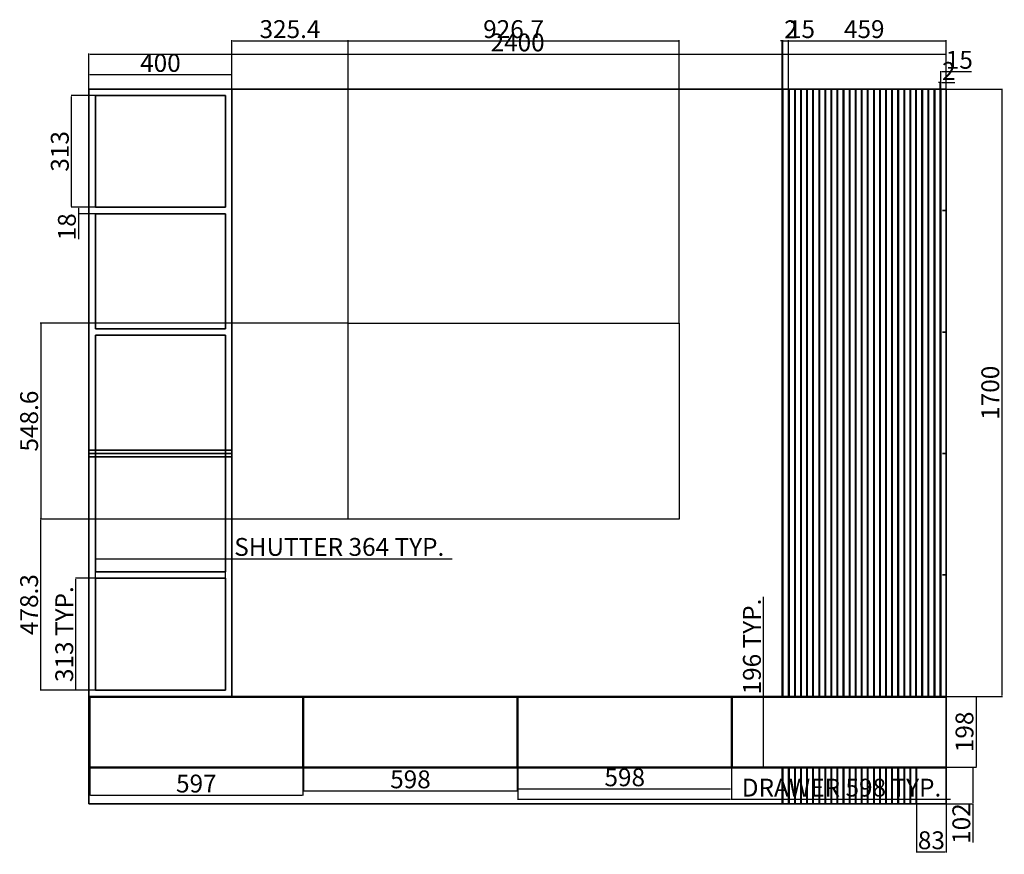
# Model space of a CAD drawing. Units: millimetres. Extents: x 805 to 3562, y 495 to 2830.
import ezdxf

# ---------------------------------------------------------------- set-up
doc = ezdxf.new("R2010")
doc.units = ezdxf.units.MM
for name, color, linetype, lineweight in [('A-ANNO-DIMS', 2, 'Continuous', 18), ('A-EQPM', 8, 'Continuous', 25), ('A-FURN', 7, 'Continuous', 35), ('A-FURN-PATT', 8, 'Continuous', 13)]:
    doc.layers.add(name, color=color, linetype=linetype, lineweight=lineweight)
doc.styles.get("Standard").update_dxf_attribs({"font": 'arial.ttf'})
doc.dimstyles.new('ISO-25', dxfattribs={"dimtxt": 50, "dimasz": 2.5, "dimexe": 1.25, "dimexo": 0.625, "dimtad": 1, "dimtxsty": 'Standard', "dimcen": 2.5, "dimadec": 0, "dimazin": 0, "dimtfac": 1, "dimtmove": 0, "dimatfit": 3, "dimfxl": 1, "dimarcsym": 0})

# ---------------------------------------------------------------- blocks, each defined once
blk = doc.blocks.new('*D1')
at = {"layer": 'A-ANNO-DIMS', "color": 0, "lineweight": -2, "transparency": 16777216}
for p, q in [((999, 2637.1), (999, 2735.5)), ((1001.5, 2734.2), (3396.5, 2734.2)), ((3399, 2637.1), (3399, 2735.5))]:
    blk.add_line(p, q, dxfattribs=at)
at = {"layer": 'A-ANNO-DIMS', "color": 0, "transparency": 16777216}
for points in [[(1001.5, 2734.6), (1001.5, 2733.8), (999, 2734.2)], [(3396.5, 2734.6), (3396.5, 2733.8), (3399, 2734.2)]]:
    blk.add_solid(points, dxfattribs=at)
at = {"layer": 'Defpoints', "color": 0, "transparency": 16777216}
for p in [(3399, 2734.2), (999, 2636.4), (3399, 2636.4)]:
    blk.add_point(p, dxfattribs=at)
at = {"layer": 'A-ANNO-DIMS', "color": 0, "transparency": 16777216, "insert": (2199, 2760.4), "char_height": 50, "attachment_point": 5}
blk.add_mtext('2400', dxfattribs=at)
blk = doc.blocks.new('*D2')
at = {"layer": 'A-ANNO-DIMS', "color": 0, "lineweight": -2, "transparency": 16777216}
for p, q in [((3384, 2637.1), (3384, 2686.8)), ((3386.5, 2685.6), (3396.5, 2685.6)), ((3399, 2637.1), (3399, 2686.8)), ((3399, 2685.6), (3470, 2685.6))]:
    blk.add_line(p, q, dxfattribs=at)
at = {"layer": 'A-ANNO-DIMS', "color": 0, "transparency": 16777216}
for points in [[(3386.5, 2686), (3386.5, 2685.1), (3384, 2685.6)], [(3396.5, 2686), (3396.5, 2685.1), (3399, 2685.6)]]:
    blk.add_solid(points, dxfattribs=at)
at = {"layer": 'Defpoints', "color": 0, "transparency": 16777216}
for p in [(3399, 2685.6), (3384, 2636.4), (3399, 2636.4)]:
    blk.add_point(p, dxfattribs=at)
at = {"layer": 'A-ANNO-DIMS', "color": 0, "transparency": 16777216, "insert": (3435.7, 2711.7), "char_height": 50, "attachment_point": 5}
blk.add_mtext('15', dxfattribs=at)
blk = doc.blocks.new('*D3')
at = {"layer": 'A-ANNO-DIMS', "color": 0, "lineweight": -2, "transparency": 16777216}
for p, q in [((3379.5, 2654.8), (3377, 2654.8)), ((3382, 2637.1), (3382, 2656.1)), ((3382, 2654.8), (3384, 2654.8)), ((3384, 2637.1), (3384, 2656.1)), ((3386.5, 2654.8), (3423.3, 2654.8))]:
    blk.add_line(p, q, dxfattribs=at)
at = {"layer": 'A-ANNO-DIMS', "color": 0, "transparency": 16777216}
for points in [[(3379.5, 2655.2), (3379.5, 2654.4), (3382, 2654.8)], [(3386.5, 2655.2), (3386.5, 2654.4), (3384, 2654.8)]]:
    blk.add_solid(points, dxfattribs=at)
at = {"layer": 'Defpoints', "color": 0, "transparency": 16777216}
for p in [(3384, 2654.8), (3382, 2636.4), (3384, 2636.4)]:
    blk.add_point(p, dxfattribs=at)
at = {"layer": 'A-ANNO-DIMS', "color": 0, "transparency": 16777216, "insert": (3406.2, 2680.5), "char_height": 50, "attachment_point": 5}
blk.add_mtext('2', dxfattribs=at)
blk = doc.blocks.new('*D4')
at = {"layer": 'A-ANNO-DIMS', "color": 0, "lineweight": -2, "transparency": 16777216}
for p, q in [((3399.6, 2636.4), (3556.2, 2636.4)), ((3555, 2633.9), (3555, 938.9)), ((3399.6, 936.4), (3556.2, 936.4))]:
    blk.add_line(p, q, dxfattribs=at)
at = {"layer": 'A-ANNO-DIMS', "color": 0, "transparency": 16777216}
for points in [[(3554.6, 2633.9), (3555.4, 2633.9), (3555, 2636.4)], [(3554.6, 938.9), (3555.4, 938.9), (3555, 936.4)]]:
    blk.add_solid(points, dxfattribs=at)
at = {"layer": 'Defpoints', "color": 0, "transparency": 16777216}
for p in [(3399, 2636.4), (3399, 936.4), (3555, 936.4)]:
    blk.add_point(p, dxfattribs=at)
at = {"layer": 'A-ANNO-DIMS', "color": 0, "transparency": 16777216, "insert": (3528.8, 1786.4), "char_height": 50, "attachment_point": 5, "rotation": 90}
blk.add_mtext('1700', dxfattribs=at)
blk = doc.blocks.new('*D5')
at = {"layer": 'A-ANNO-DIMS', "color": 0, "lineweight": -2, "transparency": 16777216}
for p, q in [((3399.6, 936.4), (3484, 936.4)), ((3482.7, 933.9), (3482.7, 740.9)), ((3399.6, 738.4), (3484, 738.4))]:
    blk.add_line(p, q, dxfattribs=at)
at = {"layer": 'A-ANNO-DIMS', "color": 0, "transparency": 16777216}
for points in [[(3482.3, 933.9), (3483.2, 933.9), (3482.7, 936.4)], [(3482.3, 740.9), (3483.2, 740.9), (3482.7, 738.4)]]:
    blk.add_solid(points, dxfattribs=at)
at = {"layer": 'Defpoints', "color": 0, "transparency": 16777216}
for p in [(3399, 936.4), (3399, 738.4), (3482.7, 738.4)]:
    blk.add_point(p, dxfattribs=at)
at = {"layer": 'A-ANNO-DIMS', "color": 0, "transparency": 16777216, "insert": (3456.6, 837.4), "char_height": 50, "attachment_point": 5, "rotation": 90}
blk.add_mtext('198', dxfattribs=at)
blk = doc.blocks.new('*D6')
at = {"layer": 'A-ANNO-DIMS', "color": 0, "lineweight": -2, "transparency": 16777216}
for p, q in [((3399.6, 738.4), (3475.2, 738.4)), ((3473.9, 735.9), (3473.9, 638.9)), ((3399.6, 636.4), (3475.2, 636.4)), ((3473.9, 636.4), (3473.9, 527.4))]:
    blk.add_line(p, q, dxfattribs=at)
at = {"layer": 'A-ANNO-DIMS', "color": 0, "transparency": 16777216}
for points in [[(3473.5, 735.9), (3474.3, 735.9), (3473.9, 738.4)], [(3473.5, 638.9), (3474.3, 638.9), (3473.9, 636.4)]]:
    blk.add_solid(points, dxfattribs=at)
at = {"layer": 'Defpoints', "color": 0, "transparency": 16777216}
for p in [(3399, 738.4), (3399, 636.4), (3473.9, 636.4)]:
    blk.add_point(p, dxfattribs=at)
at = {"layer": 'A-ANNO-DIMS', "color": 0, "transparency": 16777216, "insert": (3447.8, 580.7), "char_height": 50, "attachment_point": 5, "rotation": 90}
blk.add_mtext('102', dxfattribs=at)
blk = doc.blocks.new('*D7')
at = {"layer": 'A-ANNO-DIMS', "color": 0, "lineweight": -2, "transparency": 16777216}
for p, q in [((999, 2637.1), (999, 2678.1)), ((1001.5, 2676.9), (1396.5, 2676.9)), ((1399, 2637.1), (1399, 2678.1))]:
    blk.add_line(p, q, dxfattribs=at)
at = {"layer": 'A-ANNO-DIMS', "color": 0, "transparency": 16777216}
for points in [[(1001.5, 2677.3), (1001.5, 2676.5), (999, 2676.9)], [(1396.5, 2677.3), (1396.5, 2676.5), (1399, 2676.9)]]:
    blk.add_solid(points, dxfattribs=at)
at = {"layer": 'Defpoints', "color": 0, "transparency": 16777216}
for p in [(1399, 2676.9), (999, 2636.4), (1399, 2636.4)]:
    blk.add_point(p, dxfattribs=at)
at = {"layer": 'A-ANNO-DIMS', "color": 0, "transparency": 16777216, "insert": (1199, 2703), "char_height": 50, "attachment_point": 5}
blk.add_mtext('400', dxfattribs=at)
blk = doc.blocks.new('*D8')
at = {"layer": 'A-ANNO-DIMS', "color": 0, "lineweight": -2, "transparency": 16777216}
for p, q in [((1016.3, 2618.4), (948.7, 2618.4)), ((949.9, 2307.9), (949.9, 2615.9)), ((1016.3, 2305.4), (948.7, 2305.4))]:
    blk.add_line(p, q, dxfattribs=at)
at = {"layer": 'A-ANNO-DIMS', "color": 0, "transparency": 16777216}
for points in [[(949.5, 2615.9), (950.3, 2615.9), (949.9, 2618.4)], [(949.5, 2307.9), (950.3, 2307.9), (949.9, 2305.4)]]:
    blk.add_solid(points, dxfattribs=at)
at = {"layer": 'Defpoints', "color": 0, "transparency": 16777216}
for p in [(949.9, 2618.4), (1017, 2618.4), (1017, 2305.4)]:
    blk.add_point(p, dxfattribs=at)
at = {"layer": 'A-ANNO-DIMS', "color": 0, "transparency": 16777216, "insert": (923.8, 2461.9), "char_height": 50, "attachment_point": 5, "rotation": 90}
blk.add_mtext('313', dxfattribs=at)
blk = doc.blocks.new('*D9')
at = {"layer": 'A-ANNO-DIMS', "color": 0, "lineweight": -2, "transparency": 16777216}
for p, q in [((1001, 737.8), (1001, 658.9)), ((1598, 737.8), (1598, 658.9)), ((1003.5, 660.1), (1595.5, 660.1))]:
    blk.add_line(p, q, dxfattribs=at)
at = {"layer": 'A-ANNO-DIMS', "color": 0, "transparency": 16777216}
for points in [[(1003.5, 660.6), (1003.5, 659.7), (1001, 660.1)], [(1595.5, 660.6), (1595.5, 659.7), (1598, 660.1)]]:
    blk.add_solid(points, dxfattribs=at)
at = {"layer": 'Defpoints', "color": 0, "transparency": 16777216}
for p in [(1001, 738.4), (1598, 738.4), (1598, 660.1)]:
    blk.add_point(p, dxfattribs=at)
at = {"layer": 'A-ANNO-DIMS', "color": 0, "transparency": 16777216, "insert": (1299.5, 686.3), "char_height": 50, "attachment_point": 5}
blk.add_mtext('597', dxfattribs=at)
blk = doc.blocks.new('*D10')
at = {"layer": 'A-ANNO-DIMS', "color": 0, "lineweight": -2, "transparency": 16777216}
for p, q in [((1600, 737.8), (1600, 670.7)), ((2198, 737.8), (2198, 670.7)), ((1602.5, 672), (2195.5, 672))]:
    blk.add_line(p, q, dxfattribs=at)
at = {"layer": 'A-ANNO-DIMS', "color": 0, "transparency": 16777216}
for points in [[(1602.5, 672.4), (1602.5, 671.6), (1600, 672)], [(2195.5, 672.4), (2195.5, 671.6), (2198, 672)]]:
    blk.add_solid(points, dxfattribs=at)
at = {"layer": 'Defpoints', "color": 0, "transparency": 16777216}
for p in [(1600, 738.4), (2198, 738.4), (2198, 672)]:
    blk.add_point(p, dxfattribs=at)
at = {"layer": 'A-ANNO-DIMS', "color": 0, "transparency": 16777216, "insert": (1899, 698.1), "char_height": 50, "attachment_point": 5}
blk.add_mtext('598', dxfattribs=at)
blk = doc.blocks.new('*D11')
at = {"layer": 'A-ANNO-DIMS', "color": 0, "lineweight": -2, "transparency": 16777216}
for p, q in [((2200, 737.8), (2200, 676.4)), ((2798, 737.8), (2798, 676.4)), ((2202.5, 677.6), (2795.5, 677.6))]:
    blk.add_line(p, q, dxfattribs=at)
at = {"layer": 'A-ANNO-DIMS', "color": 0, "transparency": 16777216}
for points in [[(2202.5, 678), (2202.5, 677.2), (2200, 677.6)], [(2795.5, 678), (2795.5, 677.2), (2798, 677.6)]]:
    blk.add_solid(points, dxfattribs=at)
at = {"layer": 'Defpoints', "color": 0, "transparency": 16777216}
for p in [(2200, 738.4), (2798, 738.4), (2798, 677.6)]:
    blk.add_point(p, dxfattribs=at)
at = {"layer": 'A-ANNO-DIMS', "color": 0, "transparency": 16777216, "insert": (2499, 703.8), "char_height": 50, "attachment_point": 5}
blk.add_mtext('598', dxfattribs=at)
blk = doc.blocks.new('*D12')
at = {"layer": 'A-ANNO-DIMS', "color": 0, "lineweight": -2, "transparency": 16777216}
for p, q in [((1016.3, 2305.4), (968.5, 2305.4)), ((969.8, 2302.9), (969.8, 2289.9)), ((1016.3, 2287.4), (968.5, 2287.4)), ((969.8, 2287.4), (969.8, 2216.7))]:
    blk.add_line(p, q, dxfattribs=at)
at = {"layer": 'A-ANNO-DIMS', "color": 0, "transparency": 16777216}
for points in [[(969.3, 2302.9), (970.2, 2302.9), (969.8, 2305.4)], [(969.3, 2289.9), (970.2, 2289.9), (969.8, 2287.4)]]:
    blk.add_solid(points, dxfattribs=at)
at = {"layer": 'Defpoints', "color": 0, "transparency": 16777216}
for p in [(1017, 2305.4), (969.8, 2287.4), (1017, 2287.4)]:
    blk.add_point(p, dxfattribs=at)
at = {"layer": 'A-ANNO-DIMS', "color": 0, "transparency": 16777216, "insert": (943.6, 2250.8), "char_height": 50, "attachment_point": 5, "rotation": 90}
blk.add_mtext('18', dxfattribs=at)
blk = doc.blocks.new('SHUTTER-364x313')
for p, q in [((0, 313), (0, 0)), ((0, 313), (364, 313)), ((364, 313), (364, 0)), ((364, 0), (0, 0))]:
    blk.add_line(p, q)
blk = doc.blocks.new('DRAWER-600')
for p, q in [((0, 196), (0, 0)), ((0, 196), (598, 196)), ((598, 196), (598, 0)), ((0, 0), (598, 0))]:
    blk.add_line(p, q)
blk = doc.blocks.new('*D15')
at = {"layer": 'A-ANNO-DIMS', "color": 0, "lineweight": -2, "transparency": 16777216}
for p, q in [((1017, 1268.1), (1017, 1323.3)), ((1381, 1268.1), (1381, 1323.3)), ((1019.5, 1322), (1378.5, 1322)), ((1381, 1322), (2016, 1322))]:
    blk.add_line(p, q, dxfattribs=at)
at = {"layer": 'A-ANNO-DIMS', "color": 0, "transparency": 16777216}
for points in [[(1019.5, 1322.4), (1019.5, 1321.6), (1017, 1322)], [(1378.5, 1322.4), (1378.5, 1321.6), (1381, 1322)]]:
    blk.add_solid(points, dxfattribs=at)
at = {"layer": 'Defpoints', "color": 0, "transparency": 16777216}
for p in [(1381, 1322), (1017, 1267.4), (1381, 1267.4)]:
    blk.add_point(p, dxfattribs=at)
at = {"layer": 'A-ANNO-DIMS', "color": 0, "transparency": 16777216, "insert": (1699.7, 1348.5), "char_height": 50, "attachment_point": 5}
blk.add_mtext('SHUTTER 364 TYP.', dxfattribs=at)
blk = doc.blocks.new('*D16')
at = {"layer": 'A-ANNO-DIMS', "color": 0, "lineweight": -2, "transparency": 16777216}
for p, q in [((1016.3, 1267.4), (961.1, 1267.4)), ((962.4, 956.9), (962.4, 1264.9)), ((1016.3, 954.4), (961.1, 954.4))]:
    blk.add_line(p, q, dxfattribs=at)
at = {"layer": 'A-ANNO-DIMS', "color": 0, "transparency": 16777216}
for points in [[(961.9, 1264.9), (962.8, 1264.9), (962.4, 1267.4)], [(961.9, 956.9), (962.8, 956.9), (962.4, 954.4)]]:
    blk.add_solid(points, dxfattribs=at)
at = {"layer": 'Defpoints', "color": 0, "transparency": 16777216}
for p in [(962.4, 1267.4), (1017, 1267.4), (1017, 954.4)]:
    blk.add_point(p, dxfattribs=at)
at = {"layer": 'A-ANNO-DIMS', "color": 0, "transparency": 16777216, "insert": (936.2, 1110.9), "char_height": 50, "attachment_point": 5, "rotation": 90}
blk.add_mtext('313 TYP.', dxfattribs=at)
blk = doc.blocks.new('*D17')
at = {"layer": 'A-ANNO-DIMS', "color": 0, "lineweight": -2, "transparency": 16777216}
for p, q in [((2200, 737.8), (2200, 647.5)), ((2798, 737.8), (2798, 647.5)), ((2202.5, 648.7), (2795.5, 648.7)), ((2798, 648.7), (3411.3, 648.7))]:
    blk.add_line(p, q, dxfattribs=at)
at = {"layer": 'A-ANNO-DIMS', "color": 0, "transparency": 16777216}
for points in [[(2202.5, 649.1), (2202.5, 648.3), (2200, 648.7)], [(2795.5, 649.1), (2795.5, 648.3), (2798, 648.7)]]:
    blk.add_solid(points, dxfattribs=at)
at = {"layer": 'Defpoints', "color": 0, "transparency": 16777216}
for p in [(2200, 738.4), (2798, 738.4), (2798, 648.7)]:
    blk.add_point(p, dxfattribs=at)
at = {"layer": 'A-ANNO-DIMS', "color": 0, "transparency": 16777216, "insert": (3105.9, 674.9), "char_height": 50, "attachment_point": 5}
blk.add_mtext('DRAWER 598 TYP.', dxfattribs=at)
blk = doc.blocks.new('*D18')
at = {"layer": 'A-ANNO-DIMS', "color": 0, "lineweight": -2, "transparency": 16777216}
for p, q in [((2887.7, 934.4), (2887.7, 1215.7)), ((2798.6, 934.4), (2888.9, 934.4)), ((2887.7, 740.9), (2887.7, 931.9)), ((2798.6, 738.4), (2888.9, 738.4))]:
    blk.add_line(p, q, dxfattribs=at)
at = {"layer": 'A-ANNO-DIMS', "color": 0, "transparency": 16777216}
for points in [[(2887.2, 931.9), (2888.1, 931.9), (2887.7, 934.4)], [(2887.2, 740.9), (2888.1, 740.9), (2887.7, 738.4)]]:
    blk.add_solid(points, dxfattribs=at)
at = {"layer": 'Defpoints', "color": 0, "transparency": 16777216}
for p in [(2798, 934.4), (2887.7, 934.4), (2798, 738.4)]:
    blk.add_point(p, dxfattribs=at)
at = {"layer": 'A-ANNO-DIMS', "color": 0, "transparency": 16777216, "insert": (2861.5, 1076.3), "char_height": 50, "attachment_point": 5, "rotation": 90}
blk.add_mtext('196 TYP.', dxfattribs=at)
blk = doc.blocks.new('*D19')
at = {"layer": 'A-ANNO-DIMS', "color": 0, "lineweight": -2, "transparency": 16777216}
for p, q in [((1724.4, 1982), (1724.4, 2772.7)), ((1726.9, 2771.4), (2648.6, 2771.4)), ((2651.1, 1982), (2651.1, 2772.7))]:
    blk.add_line(p, q, dxfattribs=at)
at = {"layer": 'A-ANNO-DIMS', "color": 0, "transparency": 16777216}
for points in [[(1726.9, 2771.8), (1726.9, 2771), (1724.4, 2771.4)], [(2648.6, 2771.8), (2648.6, 2771), (2651.1, 2771.4)]]:
    blk.add_solid(points, dxfattribs=at)
at = {"layer": 'Defpoints', "color": 0, "transparency": 16777216}
for p in [(2651.1, 2771.4), (1724.4, 1981.4), (2651.1, 1981.4)]:
    blk.add_point(p, dxfattribs=at)
at = {"layer": 'A-ANNO-DIMS', "color": 0, "transparency": 16777216, "insert": (2187.8, 2797.6), "char_height": 50, "attachment_point": 5}
blk.add_mtext('926.7', dxfattribs=at)
blk = doc.blocks.new('*D20')
at = {"layer": 'A-ANNO-DIMS', "color": 0, "lineweight": -2, "transparency": 16777216}
for p, q in [((1723.8, 1981.4), (862.7, 1981.4)), ((864, 1978.9), (864, 1435.2)), ((1723.8, 1432.7), (862.7, 1432.7))]:
    blk.add_line(p, q, dxfattribs=at)
at = {"layer": 'A-ANNO-DIMS', "color": 0, "transparency": 16777216}
for points in [[(863.5, 1978.9), (864.4, 1978.9), (864, 1981.4)], [(863.5, 1435.2), (864.4, 1435.2), (864, 1432.7)]]:
    blk.add_solid(points, dxfattribs=at)
at = {"layer": 'Defpoints', "color": 0, "transparency": 16777216}
for p in [(1724.4, 1981.4), (864, 1432.7), (1724.4, 1432.7)]:
    blk.add_point(p, dxfattribs=at)
at = {"layer": 'A-ANNO-DIMS', "color": 0, "transparency": 16777216, "insert": (837.8, 1707.1), "char_height": 50, "attachment_point": 5, "rotation": 90}
blk.add_mtext('548.6', dxfattribs=at)
blk = doc.blocks.new('*D21')
at = {"layer": 'A-ANNO-DIMS', "color": 0, "lineweight": -2, "transparency": 16777216}
for p, q in [((1399, 2637.1), (1399, 2772.7)), ((1401.5, 2771.4), (1721.9, 2771.4)), ((1724.4, 1982), (1724.4, 2772.7))]:
    blk.add_line(p, q, dxfattribs=at)
at = {"layer": 'A-ANNO-DIMS', "color": 0, "transparency": 16777216}
for points in [[(1401.5, 2771.8), (1401.5, 2771), (1399, 2771.4)], [(1721.9, 2771.8), (1721.9, 2771), (1724.4, 2771.4)]]:
    blk.add_solid(points, dxfattribs=at)
at = {"layer": 'Defpoints', "color": 0, "transparency": 16777216}
for p in [(1724.4, 2771.4), (1399, 2636.4), (1724.4, 1981.4)]:
    blk.add_point(p, dxfattribs=at)
at = {"layer": 'A-ANNO-DIMS', "color": 0, "transparency": 16777216, "insert": (1561.7, 2797.6), "char_height": 50, "attachment_point": 5}
blk.add_mtext('325.4', dxfattribs=at)
blk = doc.blocks.new('*D22')
at = {"layer": 'A-ANNO-DIMS', "color": 0, "lineweight": -2, "transparency": 16777216}
for p, q in [((1723.8, 1432.7), (862.7, 1432.7)), ((864, 956.9), (864, 1430.2)), ((1380.3, 954.4), (862.7, 954.4))]:
    blk.add_line(p, q, dxfattribs=at)
at = {"layer": 'A-ANNO-DIMS', "color": 0, "transparency": 16777216}
for points in [[(863.5, 1430.2), (864.4, 1430.2), (864, 1432.7)], [(863.5, 956.9), (864.4, 956.9), (864, 954.4)]]:
    blk.add_solid(points, dxfattribs=at)
at = {"layer": 'Defpoints', "color": 0, "transparency": 16777216}
for p in [(864, 1432.7), (1724.4, 1432.7), (1381, 954.4)]:
    blk.add_point(p, dxfattribs=at)
at = {"layer": 'A-ANNO-DIMS', "color": 0, "transparency": 16777216, "insert": (837.8, 1193.6), "char_height": 50, "attachment_point": 5, "rotation": 90}
blk.add_mtext('478.3', dxfattribs=at)
blk = doc.blocks.new('*D23')
at = {"layer": 'A-ANNO-DIMS', "color": 0, "lineweight": -2, "transparency": 16777216}
for p, q in [((2940, 937.1), (2940, 2772.7)), ((2942.5, 2771.4), (3396.5, 2771.4)), ((3399, 937.1), (3399, 2772.7))]:
    blk.add_line(p, q, dxfattribs=at)
at = {"layer": 'A-ANNO-DIMS', "color": 0, "transparency": 16777216}
for points in [[(2942.5, 2771.8), (2942.5, 2771), (2940, 2771.4)], [(3396.5, 2771.8), (3396.5, 2771), (3399, 2771.4)]]:
    blk.add_solid(points, dxfattribs=at)
at = {"layer": 'Defpoints', "color": 0, "transparency": 16777216}
for p in [(3399, 2771.4), (2940, 936.4), (3399, 936.4)]:
    blk.add_point(p, dxfattribs=at)
at = {"layer": 'A-ANNO-DIMS', "color": 0, "transparency": 16777216, "insert": (3169.5, 2797.6), "char_height": 50, "attachment_point": 5}
blk.add_mtext('459', dxfattribs=at)
blk = doc.blocks.new('*D24')
at = {"layer": 'A-ANNO-DIMS', "color": 0, "lineweight": -2, "transparency": 16777216}
for p, q in [((2937.5, 2771.4), (2935, 2771.4)), ((2940, 2637.1), (2940, 2772.7)), ((2940, 2771.4), (2942, 2771.4)), ((2942, 2637.1), (2942, 2772.7)), ((2944.5, 2771.4), (2981.3, 2771.4))]:
    blk.add_line(p, q, dxfattribs=at)
at = {"layer": 'A-ANNO-DIMS', "color": 0, "transparency": 16777216}
for points in [[(2937.5, 2771.8), (2937.5, 2771), (2940, 2771.4)], [(2944.5, 2771.8), (2944.5, 2771), (2942, 2771.4)]]:
    blk.add_solid(points, dxfattribs=at)
at = {"layer": 'Defpoints', "color": 0, "transparency": 16777216}
for p in [(2942, 2771.4), (2940, 2636.4), (2942, 2636.4)]:
    blk.add_point(p, dxfattribs=at)
at = {"layer": 'A-ANNO-DIMS', "color": 0, "transparency": 16777216, "insert": (2964.2, 2797.2), "char_height": 50, "attachment_point": 5}
blk.add_mtext('2', dxfattribs=at)
blk = doc.blocks.new('*D25')
at = {"layer": 'A-ANNO-DIMS', "color": 0, "lineweight": -2, "transparency": 16777216}
for p, q in [((2942, 2637.1), (2942, 2772.7)), ((2944.5, 2771.4), (2954.5, 2771.4)), ((2957, 2637.1), (2957, 2772.7)), ((2957, 2771.4), (3028, 2771.4))]:
    blk.add_line(p, q, dxfattribs=at)
at = {"layer": 'A-ANNO-DIMS', "color": 0, "transparency": 16777216}
for points in [[(2944.5, 2771.8), (2944.5, 2771), (2942, 2771.4)], [(2954.5, 2771.8), (2954.5, 2771), (2957, 2771.4)]]:
    blk.add_solid(points, dxfattribs=at)
at = {"layer": 'Defpoints', "color": 0, "transparency": 16777216}
for p in [(2957, 2771.4), (2942, 2636.4), (2957, 2636.4)]:
    blk.add_point(p, dxfattribs=at)
at = {"layer": 'A-ANNO-DIMS', "color": 0, "transparency": 16777216, "insert": (2993.7, 2797.6), "char_height": 50, "attachment_point": 5}
blk.add_mtext('15', dxfattribs=at)
blk = doc.blocks.new('*D26')
at = {"layer": 'A-ANNO-DIMS', "color": 0, "lineweight": -2, "transparency": 16777216}
for p, q in [((3316, 635.8), (3316, 500.2)), ((3399, 635.8), (3399, 500.2)), ((3318.5, 501.4), (3396.5, 501.4))]:
    blk.add_line(p, q, dxfattribs=at)
at = {"layer": 'A-ANNO-DIMS', "color": 0, "transparency": 16777216}
for points in [[(3318.5, 501.8), (3318.5, 501), (3316, 501.4)], [(3396.5, 501.8), (3396.5, 501), (3399, 501.4)]]:
    blk.add_solid(points, dxfattribs=at)
at = {"layer": 'Defpoints', "color": 0, "transparency": 16777216}
for p in [(3316, 636.4), (3399, 636.4), (3399, 501.4)]:
    blk.add_point(p, dxfattribs=at)
at = {"layer": 'A-ANNO-DIMS', "color": 0, "transparency": 16777216, "insert": (3357.5, 527.6), "char_height": 50, "attachment_point": 5}
blk.add_mtext('83', dxfattribs=at)

msp = doc.modelspace()

# ---------------------------------------------------------------- linework, layer by layer
at = {"layer": 'A-EQPM'}
msp.add_lwpolyline([(1724.397, 1981.371), (2651.128, 1981.371), (2651.128, 1432.748), (1724.397, 1432.748)], close=True, dxfattribs=at)
at = {"layer": 'A-FURN'}
for p, q in [((3398.966, 2636.428), (998.966, 2636.428)), ((998.966, 2636.428), (998.966, 636.428)), ((998.966, 2636.428), (1398.966, 2636.428)), ((1398.966, 2636.428), (1398.966, 936.428)), ((2939.966, 936.428), (2939.966, 2636.428)), ((2941.966, 936.428), (2941.966, 2636.428)), ((2958.966, 936.428), (2958.966, 2636.428)), ((2975.966, 936.428), (2975.966, 2636.428)), ((2992.966, 936.428), (2992.966, 2636.428)), ((3009.966, 936.428), (3009.966, 2636.428)), ((3026.966, 936.428), (3026.966, 2636.428)), ((3043.966, 936.428), (3043.966, 2636.428)), ((3060.966, 936.428), (3060.966, 2636.428)), ((3077.966, 936.428), (3077.966, 2636.428)), ((3094.966, 936.428), (3094.966, 2636.428)), ((3111.966, 936.428), (3111.966, 2636.428)), ((3128.966, 936.428), (3128.966, 2636.428)), ((3145.966, 936.428), (3145.966, 2636.428)), ((3162.966, 936.428), (3162.966, 2636.428)), ((3179.966, 936.428), (3179.966, 2636.428)), ((3196.966, 936.428), (3196.966, 2636.428)), ((3213.966, 936.428), (3213.966, 2636.428)), ((3230.966, 936.428), (3230.966, 2636.428)), ((3247.966, 936.428), (3247.966, 2636.428)), ((3264.966, 936.428), (3264.966, 2636.428)), ((3281.966, 936.428), (3281.966, 2636.428)), ((3298.966, 936.428), (3298.966, 2636.428)), ((3313.966, 936.428), (3313.966, 2636.428)), ((3313.966, 936.428), (3313.966, 2636.428)), ((3313.966, 936.428), (3313.966, 2636.428)), ((3330.966, 936.428), (3330.966, 2636.428)), ((3332.966, 936.428), (3332.966, 2636.428)), ((3364.966, 936.428), (3364.966, 2636.428)), ((3366.966, 936.428), (3366.966, 2636.428)), ((3381.966, 936.428), (3381.966, 2636.428)), ((3383.966, 936.428), (3383.966, 2636.428)), ((3398.966, 636.428), (3398.966, 2636.428)), ((3398.966, 2296.428), (3388.966, 2296.428)), ((3398.966, 2296.428), (3388.966, 2296.428)), ((1380.966, 2287.428), (1016.966, 2287.428)), ((1016.966, 2287.428), (1016.966, 1965.428)), ((1380.966, 2287.428), (1380.966, 1965.428)), ((1380.966, 1965.428), (1016.966, 1965.428)), ((1380.966, 1947.428), (1016.966, 1947.428)), ((1016.966, 1947.428), (1016.966, 1285.428)), ((1380.966, 1947.428), (1380.966, 1285.428)), ((3398.966, 1956.428), (3388.966, 1956.428)), ((3398.966, 1956.428), (3388.966, 1956.428)), ((1398.966, 1625.428), (998.966, 1625.428)), ((1398.966, 1616.428), (998.966, 1616.428)), ((1398.966, 1616.428), (998.966, 1616.428)), ((1398.966, 1607.428), (998.966, 1607.428)), ((3398.966, 1616.428), (3388.966, 1616.428)), ((3398.966, 1616.428), (3388.966, 1616.428)), ((1380.966, 1285.428), (1016.966, 1285.428)), ((3398.966, 1276.428), (3388.966, 1276.428)), ((998.966, 936.428), (998.966, 736.428)), ((1016.966, 936.428), (998.966, 936.428)), ((1016.966, 934.428), (1000.966, 934.428)), ((1000.966, 934.428), (1000.966, 738.428)), ((1016.966, 936.428), (3398.966, 936.428)), ((1016.966, 936.428), (1398.966, 936.428)), ((1016.966, 934.428), (1597.966, 934.428)), ((1597.966, 934.428), (1597.966, 738.428)), ((2799.966, 934.428), (2799.966, 738.428)), ((2799.966, 934.428), (3398.966, 934.428)), ((998.966, 736.428), (3398.966, 736.428)), ((1000.966, 738.428), (1597.966, 738.428)), ((2799.966, 738.428), (3398.966, 738.428)), ((2939.966, 636.428), (2939.966, 736.428)), ((2941.966, 636.428), (2941.966, 736.428)), ((2958.966, 636.428), (2958.966, 736.428)), ((2975.966, 636.428), (2975.966, 736.428)), ((2992.966, 636.428), (2992.966, 736.428)), ((3009.966, 636.428), (3009.966, 736.428)), ((3026.966, 636.428), (3026.966, 736.428)), ((3043.966, 636.428), (3043.966, 736.428)), ((3060.966, 636.428), (3060.966, 736.428)), ((3077.966, 636.428), (3077.966, 736.428)), ((3094.966, 636.428), (3094.966, 736.428)), ((3111.966, 636.428), (3111.966, 736.428)), ((3128.966, 636.428), (3128.966, 736.428)), ((3145.966, 636.428), (3145.966, 736.428)), ((3162.966, 636.428), (3162.966, 736.428)), ((3179.966, 636.428), (3179.966, 736.428)), ((3196.966, 636.428), (3196.966, 736.428)), ((3213.966, 636.428), (3213.966, 736.428)), ((3230.966, 636.428), (3230.966, 736.428)), ((3247.966, 636.428), (3247.966, 736.428)), ((3264.966, 636.428), (3264.966, 736.428)), ((3281.966, 636.428), (3281.966, 736.428)), ((3298.966, 636.428), (3298.966, 736.428)), ((3315.966, 636.428), (3315.966, 736.428)), ((998.966, 636.428), (3398.966, 636.428))]:
    msp.add_line(p, q, dxfattribs=at)
at = {"layer": 'A-FURN-PATT'}
for p, q in [((2956.966, 936.428), (2956.966, 2636.428)), ((2956.966, 936.428), (2956.966, 2636.428)), ((2973.966, 936.428), (2973.966, 2636.428)), ((2973.966, 936.428), (2973.966, 2636.428)), ((2990.966, 936.428), (2990.966, 2636.428)), ((2990.966, 936.428), (2990.966, 2636.428)), ((3007.966, 936.428), (3007.966, 2636.428)), ((3007.966, 936.428), (3007.966, 2636.428)), ((3024.966, 936.428), (3024.966, 2636.428)), ((3024.966, 936.428), (3024.966, 2636.428)), ((3041.966, 936.428), (3041.966, 2636.428)), ((3041.966, 936.428), (3041.966, 2636.428)), ((3058.966, 936.428), (3058.966, 2636.428)), ((3058.966, 936.428), (3058.966, 2636.428)), ((3075.966, 936.428), (3075.966, 2636.428)), ((3075.966, 936.428), (3075.966, 2636.428)), ((3092.966, 936.428), (3092.966, 2636.428)), ((3092.966, 936.428), (3092.966, 2636.428)), ((3109.966, 936.428), (3109.966, 2636.428)), ((3109.966, 936.428), (3109.966, 2636.428)), ((3126.966, 936.428), (3126.966, 2636.428)), ((3126.966, 936.428), (3126.966, 2636.428)), ((3143.966, 936.428), (3143.966, 2636.428)), ((3143.966, 936.428), (3143.966, 2636.428)), ((3160.966, 936.428), (3160.966, 2636.428)), ((3160.966, 936.428), (3160.966, 2636.428)), ((3177.966, 936.428), (3177.966, 2636.428)), ((3177.966, 936.428), (3177.966, 2636.428)), ((3194.966, 936.428), (3194.966, 2636.428)), ((3194.966, 936.428), (3194.966, 2636.428)), ((3211.966, 936.428), (3211.966, 2636.428)), ((3211.966, 936.428), (3211.966, 2636.428)), ((3228.966, 936.428), (3228.966, 2636.428)), ((3228.966, 936.428), (3228.966, 2636.428)), ((3245.966, 936.428), (3245.966, 2636.428)), ((3245.966, 936.428), (3245.966, 2636.428)), ((3262.966, 936.428), (3262.966, 2636.428)), ((3262.966, 936.428), (3262.966, 2636.428)), ((3279.966, 936.428), (3279.966, 2636.428)), ((3279.966, 936.428), (3279.966, 2636.428)), ((3296.966, 936.428), (3296.966, 2636.428)), ((3296.966, 936.428), (3296.966, 2636.428)), ((3315.966, 936.428), (3315.966, 2636.428)), ((3315.966, 936.428), (3315.966, 2636.428)), ((3347.966, 936.428), (3347.966, 2636.428)), ((3347.966, 936.428), (3347.966, 2636.428)), ((3349.966, 936.428), (3349.966, 2636.428)), ((3349.966, 936.428), (3349.966, 2636.428)), ((2956.966, 636.428), (2956.966, 736.428)), ((2956.966, 636.428), (2956.966, 736.428)), ((2973.966, 636.428), (2973.966, 736.428)), ((2973.966, 636.428), (2973.966, 736.428)), ((2990.966, 636.428), (2990.966, 736.428)), ((2990.966, 636.428), (2990.966, 736.428)), ((3007.966, 636.428), (3007.966, 736.428)), ((3007.966, 636.428), (3007.966, 736.428)), ((3024.966, 636.428), (3024.966, 736.428)), ((3024.966, 636.428), (3024.966, 736.428)), ((3041.966, 636.428), (3041.966, 736.428)), ((3041.966, 636.428), (3041.966, 736.428)), ((3058.966, 636.428), (3058.966, 736.428)), ((3058.966, 636.428), (3058.966, 736.428)), ((3075.966, 636.428), (3075.966, 736.428)), ((3075.966, 636.428), (3075.966, 736.428)), ((3092.966, 636.428), (3092.966, 736.428)), ((3092.966, 636.428), (3092.966, 736.428)), ((3109.966, 636.428), (3109.966, 736.428)), ((3109.966, 636.428), (3109.966, 736.428)), ((3126.966, 636.428), (3126.966, 736.428)), ((3126.966, 636.428), (3126.966, 736.428)), ((3143.966, 636.428), (3143.966, 736.428)), ((3143.966, 636.428), (3143.966, 736.428)), ((3160.966, 636.428), (3160.966, 736.428)), ((3160.966, 636.428), (3160.966, 736.428)), ((3177.966, 636.428), (3177.966, 736.428)), ((3177.966, 636.428), (3177.966, 736.428)), ((3194.966, 636.428), (3194.966, 736.428)), ((3194.966, 636.428), (3194.966, 736.428)), ((3211.966, 636.428), (3211.966, 736.428)), ((3211.966, 636.428), (3211.966, 736.428)), ((3228.966, 636.428), (3228.966, 736.428)), ((3228.966, 636.428), (3228.966, 736.428)), ((3245.966, 636.428), (3245.966, 736.428)), ((3245.966, 636.428), (3245.966, 736.428)), ((3262.966, 636.428), (3262.966, 736.428)), ((3262.966, 636.428), (3262.966, 736.428)), ((3279.966, 636.428), (3279.966, 736.428)), ((3279.966, 636.428), (3279.966, 736.428)), ((3296.966, 636.428), (3296.966, 736.428)), ((3296.966, 636.428), (3296.966, 736.428)), ((3313.966, 636.428), (3313.966, 736.428)), ((3313.966, 636.428), (3313.966, 736.428))]:
    msp.add_line(p, q, dxfattribs=at)

# ---------------------------------------------------------------- block references
at = {"layer": 'A-FURN'}
for name, p in [('SHUTTER-364x313', (1016.966, 2305.428)), ('SHUTTER-364x313', (1016.966, 954.428)), ('DRAWER-600', (1599.966, 738.428)), ('DRAWER-600', (2199.966, 738.428))]:
    msp.add_blockref(name, p, dxfattribs=at)

# ---------------------------------------------------------------- dimensions: what is measured, and where the dimension line sits
at = {"layer": 'A-ANNO-DIMS'}
for base, p1, p2, override, picture, middle in [((1724.397, 2771.428), (1398.966, 2636.428), (1724.397, 1981.371), {"dimdec": 1, "dimlfac": 1, "dimrnd": 0, "dimzin": 0, "dimdsep": 46, "dimlunit": 2}, '*D21', (1561.682, 2797.599)), ((2651.128, 2771.428), (1724.397, 1981.371), (2651.128, 1981.371), {"dimdec": 1, "dimlfac": 1, "dimrnd": 0, "dimzin": 0, "dimdsep": 46, "dimlunit": 2}, '*D19', (2187.763, 2797.582)), ((2941.966, 2771.428), (2939.966, 2636.428), (2941.966, 2636.428), {"dimdec": 0, "dimlfac": 1, "dimrnd": 0, "dimzin": 0, "dimdsep": 46, "dimlunit": 2}, '*D24', (2964.15, 2797.156)), ((3398.966, 2771.428), (2939.966, 936.428), (3398.966, 936.428), {"dimdec": 0, "dimlfac": 1, "dimrnd": 0, "dimzin": 0, "dimdsep": 46, "dimlunit": 2}, '*D23', (3169.466, 2797.582)), ((2956.966, 2771.428), (2941.966, 2636.428), (2956.966, 2636.428), {"dimdec": 0, "dimlfac": 1, "dimrnd": 0, "dimzin": 0, "dimdsep": 46, "dimlunit": 2}, '*D25', (2993.737, 2797.582)), ((3398.966, 2734.221), (998.966, 2636.428), (3398.966, 2636.428), {"dimclrd": 0, "dimclre": 0, "dimclrt": 0}, '*D1', (2198.966, 2760.375)), ((1398.966, 2676.886), (998.966, 2636.428), (1398.966, 2636.428), {"dimclrd": 0, "dimclre": 0, "dimclrt": 0}, '*D7', (1198.966, 2703.039)), ((3398.966, 2685.565), (3383.966, 2636.428), (3398.966, 2636.428), {"dimclrd": 0, "dimclre": 0, "dimclrt": 0}, '*D2', (3435.737, 2711.719)), ((3383.966, 2654.801), (3381.966, 2636.428), (3383.966, 2636.428), {"dimclrd": 0, "dimclre": 0, "dimclrt": 0}, '*D3', (3406.15, 2680.529)), ((1597.966, 660.141), (1000.966, 738.428), (1597.966, 738.428), {"dimclrd": 0, "dimclre": 0, "dimclrt": 0}, '*D9', (1299.466, 686.295)), ((2197.966, 671.981), (1599.966, 738.428), (2197.966, 738.428), {"dimclrd": 0, "dimclre": 0, "dimclrt": 0}, '*D10', (1898.966, 698.135)), ((2797.966, 677.617), (2199.966, 738.428), (2797.966, 738.428), {"dimclrd": 0, "dimclre": 0, "dimclrt": 0}, '*D11', (2498.966, 703.771)), ((3398.966, 501.428), (3315.966, 636.428), (3398.966, 636.428), {"dimdec": 0, "dimlfac": 1, "dimrnd": 0, "dimzin": 0, "dimdsep": 46, "dimlunit": 2}, '*D26', (3357.466, 527.599))]:
    dim = msp.add_linear_dim(base=base, p1=p1, p2=p2, dimstyle='ISO-25', override=override, dxfattribs=at)
    dim.commit()
    dim.dimension.update_dxf_attribs({"geometry": picture, "text_midpoint": middle})
for base, p1, p2, override, picture, middle in [((3554.989, 936.428), (3398.966, 2636.428), (3398.966, 936.428), {"dimclrd": 0, "dimclre": 0, "dimclrt": 0}, '*D4', (3528.835, 1786.428)), ((949.922, 2618.428), (1016.966, 2305.428), (1016.966, 2618.428), {"dimclrd": 0, "dimclre": 0, "dimclrt": 0}, '*D8', (923.751, 2461.928)), ((969.753, 2287.428), (1016.966, 2305.428), (1016.966, 2287.428), {"dimclrd": 0, "dimclre": 0, "dimclrt": 0}, '*D12', (943.599, 2250.794)), ((863.966, 1432.748), (1724.397, 1981.371), (1724.397, 1432.748), {"dimdec": 1, "dimlfac": 1, "dimrnd": 0, "dimzin": 0, "dimdsep": 46, "dimlunit": 2}, '*D20', (837.813, 1707.059)), ((863.966, 1432.748), (1380.966, 954.428), (1724.397, 1432.748), {"dimdec": 1, "dimlfac": 1, "dimrnd": 0, "dimzin": 0, "dimdsep": 46, "dimlunit": 2}, '*D22', (837.796, 1193.588)), ((3482.74, 738.428), (3398.966, 936.428), (3398.966, 738.428), {"dimclrd": 0, "dimclre": 0, "dimclrt": 0}, '*D5', (3456.587, 837.428)), ((3473.929, 636.428), (3398.966, 738.428), (3398.966, 636.428), {"dimclrd": 0, "dimclre": 0, "dimclrt": 0}, '*D6', (3447.775, 580.677))]:
    dim = msp.add_linear_dim(base=base, p1=p1, p2=p2, angle=90, dimstyle='ISO-25', override=override, dxfattribs=at)
    dim.commit()
    dim.dimension.update_dxf_attribs({"geometry": picture, "text_midpoint": middle})
for base, p1, p2, text, picture, middle in [((1380.966, 1322.028), (1016.966, 1267.428), (1380.966, 1267.428), 'SHUTTER <> TYP.', '*D15', (1699.712, 1348.523)), ((2797.966, 648.728), (2199.966, 738.428), (2797.966, 738.428), 'DRAWER <> TYP.', '*D17', (3105.883, 674.882))]:
    dim = msp.add_linear_dim(base=base, p1=p1, p2=p2, text=text, dimstyle='ISO-25', override={"dimdec": 0, "dimlfac": 1, "dimrnd": 0, "dimzin": 0, "dimdsep": 46, "dimlunit": 2}, dxfattribs=at)
    dim.commit()
    dim.dimension.update_dxf_attribs({"geometry": picture, "text_midpoint": middle})
for base, p1, p2, picture, middle in [((962.366, 1267.428), (1016.966, 954.428), (1016.966, 1267.428), '*D16', (936.196, 1110.928)), ((2887.666, 934.428), (2797.966, 738.428), (2797.966, 934.428), '*D18', (2861.513, 1076.315))]:
    dim = msp.add_linear_dim(base=base, p1=p1, p2=p2, angle=90, text='<> TYP.', dimstyle='ISO-25', override={"dimdec": 0, "dimlfac": 1, "dimrnd": 0, "dimzin": 0, "dimdsep": 46, "dimlunit": 2}, dxfattribs=at)
    dim.commit()
    dim.dimension.update_dxf_attribs({"geometry": picture, "text_midpoint": middle})

doc.saveas('drawing.dxf')
